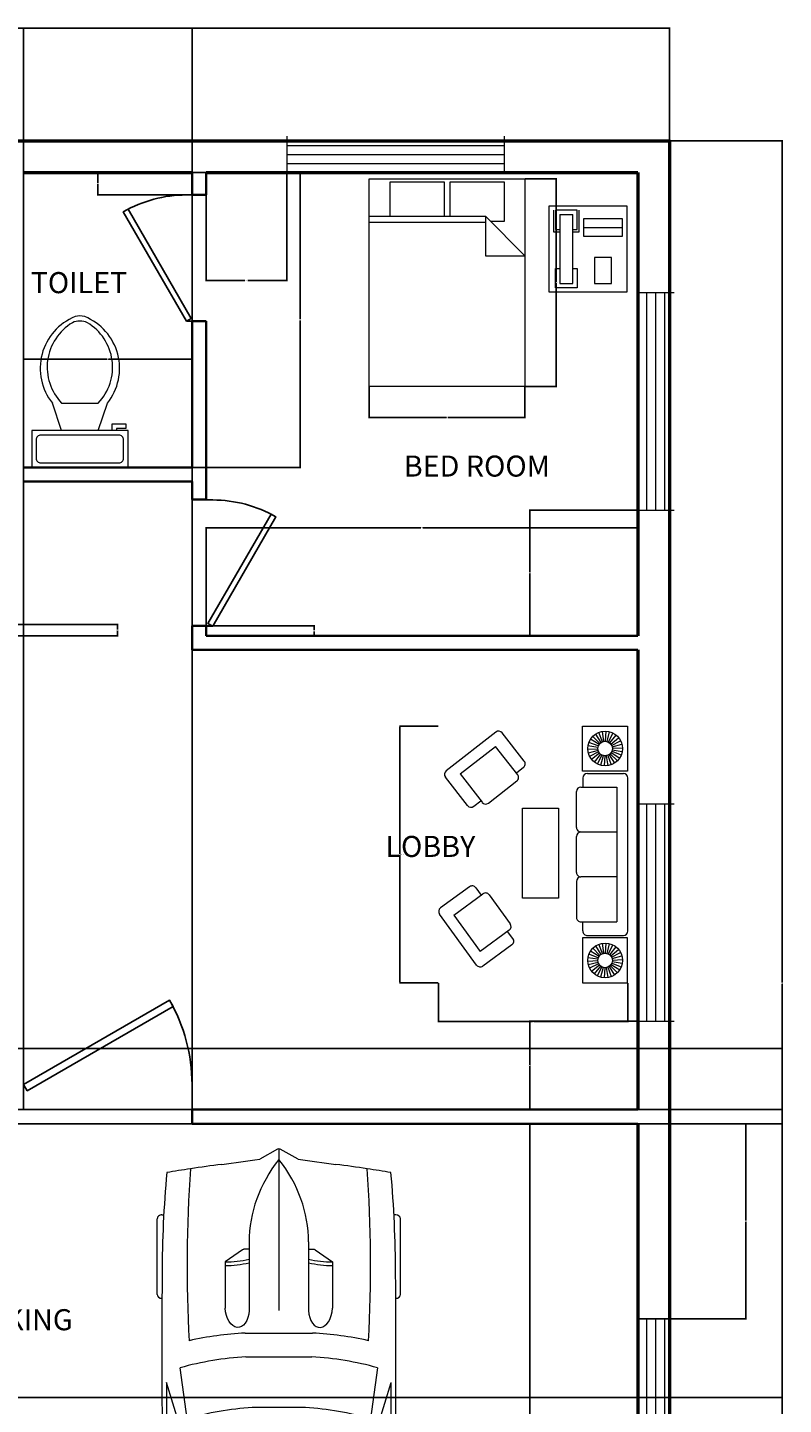
# Model space of a CAD drawing. Units: feet. Extents: x 3746 to 4170, y 1475 to 2148.
# Tile 5 of 5: x 3955 to 4170, y 1755 to 2148. Entities that reach past the tile are written whole.
import ezdxf

# ---------------------------------------------------------------- set-up
doc = ezdxf.new("R2010")
doc.units = ezdxf.units.FT
for name, color, linetype, lineweight in [('A-ANNO-DIMS', 2, 'Continuous', 18), ('A-AREA-IDEN', 7, 'Continuous', 25), ('A-EQPM', 8, 'Continuous', 13), ('A-FLOR-FIXT', 9, 'Continuous', 18), ('A-GLAZ', 91, 'Continuous', 18), ('CAR', 20, 'Continuous', 13), ('DOOR', 135, 'Continuous', 25), ('FURNITURE', 43, 'Continuous', 18), ('INWER WALL', 30, 'Continuous', 35), ('OUTER WALL', 31, 'Continuous', 50)]:
    doc.layers.add(name, color=color, linetype=linetype, lineweight=lineweight)
doc.styles.get("Standard").update_dxf_attribs({"font": 'arial.ttf'})
doc.dimstyles.get("Standard").update_dxf_attribs({"dimtxt": 0.18, "dimasz": 0.18, "dimexe": 0.18, "dimexo": 0.0625, "dimgap": 0.09, "dimtad": 0, "dimtih": 1, "dimtoh": 1, "dimdec": 4, "dimzin": 0, "dimdsep": 46, "dimtxsty": 'Standard', "dimcen": 0.09, "dimadec": 0, "dimazin": 0, "dimtfac": 1, "dimtdec": 4, "dimtofl": 0, "dimtmove": 0, "dimatfit": 3, "dimfxl": 1, "dimtolj": 1, "dimtzin": 0, "dimarcsym": 0})

# ---------------------------------------------------------------- blocks, each defined once
blk = doc.blocks.new('*U2')
for p, q in [((0, 0), (0, -6)), ((40, 0), (40, -6))]:
    blk.add_line(p, q)
blk.add_lwpolyline([(0, 0), (34.64, 20), (35.52, 18.48), (0.87, -1.52)], close=True)
blk.add_arc((0, 0), 40, 0, 30)
blk = doc.blocks.new('*U3')
for p, q in [((0, 0), (0, 6)), ((40, 0), (40, 6))]:
    blk.add_line(p, q)
blk.add_lwpolyline([(0, 0), (34.64, -20), (35.52, -18.48), (0.87, 1.52)], close=True)
blk.add_arc((0, 0), 40, 330, 0)
blk = doc.blocks.new('Bed - Queen')
for p, q in [((0, -80.00003), (0, 0)), ((0, 0), (59.99999, 0)), ((59.99999, 0), (59.99999, -80.00003)), ((7.99999, -1.2), (28.79998, -1.2)), ((7.99999, -14.4), (7.99999, -1.2)), ((28.79998, -1.2), (28.79998, -14.4)), ((31.19999, -1.2), (51.99999, -1.2)), ((31.19999, -14.4), (31.19999, -1.2)), ((51.99999, -1.2), (51.99999, -16.4)), ((0, -14.4), (44.8, -14.4)), ((59.99999, -29.6), (44.8, -14.4)), ((44.8, -14.4), (44.8, -29.6)), ((44.8, -16.8), (0, -16.8)), ((51.99999, -16.4), (46.79936, -16.4)), ((44.8, -29.6), (59.99999, -29.6)), ((59.99999, -80.00003), (0, -80.00003))]:
    blk.add_line(p, q)
blk = doc.blocks.new('Toilet - top')
for p, q in [((9.5, -6), (9.5, -2)), ((-10, -8.5), (-8, -8.5)), ((-10, -9.5), (-10, -8.5)), ((-8, -8.5), (-8, -8)), ((-7, -8), (-7, -9.5)), ((-4, -8), (-6, -14)), ((4, -8), (6, -14)), ((-7, -9.5), (-10, -9.5)), ((4, -14), (-4, -14))]:
    blk.add_line(p, q)
blk.add_lwpolyline([(10.5, -8), (10.5, 0), (-10.5, 0), (-10.5, -8)], close=True)
for points in [[(-9.5, -2), (-9.5, -6)], [(8.5, -1), (-8.5, -1)], [(-8.5, -7), (8.5, -7)]]:
    blk.add_lwpolyline(points)
for centre, radius, start, end in [((-8.62, -1.88), 0.884, 81.8699, 188.1301), ((8.62, -1.88), 0.884, 351.8699, 98.1301), ((-8.62, -6.12), 0.884, 171.8699, 278.1301), ((8.62, -6.12), 0.884, 261.8699, 8.1301), ((3.52, -21.58), 12.17, 141.4691, 247.9714), ((4.2, -21.82), 11.33, 136.3677, 238.9468), ((-3.52, -21.58), 12.17, 292.0284, 38.5307), ((-4.2, -21.82), 11.33, 301.053, 43.6321), ((0, -27.88), 4, 245.7318, 294.2682), ((0, -29), 4, 254.8605, 285.1395)]:
    blk.add_arc(centre, radius, start, end)
blk = doc.blocks.new('Phone - Desk')
for p, q in [((-4.5, -5), (-4.5, 5)), ((-4.5, 5), (4.5, 5)), ((4.5, 5), (4.5, -5)), ((-4, 4.5), (-4, 2)), ((-3.75, 4.5), (-3.75, 2.25)), ((-1.25, 4.5), (-3.75, 4.5)), ((-3.25, 4), (-3.25, -4)), ((-3.25, 4), (-1.75, 4)), ((-1.75, -4), (-1.75, 4)), ((-1.25, 2.25), (-1.25, 4.5)), ((-1, 2), (-1, 4.5)), ((4, 3.5), (-0.5, 3.5)), ((-0.5, 3.5), (-0.5, 1.5)), ((4, 1.5), (4, 3.5)), ((-4, 2), (-3.25, 2)), ((-3.75, 2.25), (-3.25, 2.25)), ((-1.75, 2.25), (-1.25, 2.25)), ((-1.75, 2), (-1, 2)), ((-0.5, 2.5), (4, 2.5)), ((-0.5, 1.5), (4, 1.5)), ((2.75, -1), (0.75, -1)), ((0.75, -1), (0.75, -4)), ((2.75, -4), (2.75, -1)), ((-3.75, -2.25), (-3.25, -2.25)), ((-3.75, -4.5), (-3.75, -2.25)), ((-1.75, -2.25), (-1.25, -2.25)), ((-1.25, -2.25), (-1.25, -4.5)), ((-1.25, -4.5), (-3.75, -4.5)), ((-3.25, -4), (-1.75, -4)), ((0.75, -4), (2.75, -4)), ((4.5, -5), (-4.5, -5))]:
    blk.add_line(p, q)
blk = doc.blocks.new('*U12')
for p, q in [((21.1, 37.41), (21.1, 36.83)), ((46.55, 38.89), (22.35, 38.89)), ((47.8, 37.39), (47.8, 37.41)), ((87.99, 31.87), (74.76, 35.92)), ((134.31, 35.6), (119.29, 31.78)), ((135.45, 37.07), (135.45, 37.41)), ((136.7, 38.89), (160.9, 38.89)), ((162.15, 37.41), (162.15, 36.77)), ((70.03, 31.54), (86.41, 29.35)), ((186.47, -33.5), (186.47, 33.5)), ((188.4, -32.76), (188.4, 32.76)), ((138.42, 29.35), (157.25, 29.35)), ((186.47, 29.35), (167.01, 29.35)), ((164.52, 26.39), (164.52, -26.39)), ((32.27, 11.63), (36.13, 17.17)), ((36.13, 17.17), (50.94, 17.17)), ((29.77, 9.51), (51.68, 9.51)), ((32.12, 9.51), (32.12, 11.15)), ((58.92, -10.77), (58.92, 10.77)), ((66.55, -10.53), (66.55, 10.53)), ((186.47, -10.53), (186.47, 10.53)), ((3.27, 6.13), (0.1, 0.41)), ((82.74, 8.5), (82.74, -8.5)), ((0, 0), (51.68, 0)), ((0.1, -0.41), (3.27, -6.13)), ((29.77, -9.51), (51.68, -9.51)), ((32.12, -9.51), (32.12, -11.15)), ((32.27, -11.63), (36.13, -17.17)), ((36.13, -17.17), (50.94, -17.17)), ((86.41, -29.35), (70.03, -31.54)), ((157.25, -29.35), (138.42, -29.35)), ((167.01, -29.35), (186.47, -29.35)), ((87.99, -31.87), (74.76, -35.92)), ((134.31, -35.6), (119.29, -31.78)), ((21.1, -37.41), (21.1, -36.83)), ((46.55, -38.89), (22.35, -38.89)), ((47.8, -37.39), (47.8, -37.41)), ((135.45, -37.07), (135.45, -37.41)), ((136.7, -38.89), (160.9, -38.89)), ((162.15, -37.41), (162.15, -36.77))]:
    blk.add_line(p, q)
for centre, major_axis, ratio, start_param, end_param in [((266.03, -27.52), (0, 313.31), 0.842304, 1.367076, 1.39176), ((41.19, -490.86), (0, 528.23), 0.842304, 0.00281, 0.075598), ((22.35, 37.41), (0, -1.48), 0.842304, 3.141593, 4.712389), ((64.48, -10555.62), (0, 10593.03), 0.842304, -0.013397, 0.002797), ((46.55, 37.41), (0, 1.48), 0.842304, -1.570796, 0), ((64.48, -10555.62), (0, -10591.55), 0.842304, 3.133765, 3.140441), ((136.7, 37.41), (0, -1.48), 0.842304, 3.141593, 4.712389), ((160.9, 37.41), (0, 1.48), 0.842304, -1.570796, 0), ((180.63, 35.84), (0, 2.22), 0.842304, -0.013017, 1.249894), ((64.48, -10556.36), (0, 10595.31), 0.842304, -0.013397, -0.013017), ((183.98, 33.5), (0, -2.96), 0.842304, 1.570796, 3.128196), ((183.98, 32.76), (0, -5.25), 0.842304, 1.570796, 3.128196), ((135.29, 5.39), (0, 81.77), 0.842304, 1.245306, 1.50788), ((95.79, -3666.35), (0, -3698.24), 0.842304, 3.134049, 3.144098), ((259.18, -27.52), (0, -305.3), 0.842304, 4.528606, 4.561838), ((37.47, -593.96), (0, -623.33), 0.842304, 3.096046, 3.200911), ((134.4, 5.39), (0, -89.78), 0.842304, 4.449482, 4.652344), ((149.6, 2.8), (0, -79.58), 0.842304, 4.372215, 4.640744), ((17.08, 0), (0, 147.02), 0.842304, 4.511394, 4.913384), ((35.91, 0), (0, 147.02), 0.842304, 4.511394, 4.913384), ((167.01, 26.39), (0, 2.96), 0.842304, 0, 1.570796), ((-204.49, 52.4), (0, -250.96), 0.842304, 1.385369, 1.434372), ((13.04, 17.01), (0, 27.42), 0.842304, 4.435146, 4.718221), ((14.2, 17.01), (0, 27.42), 0.842304, 4.435146, 4.718221), ((50.79, 13.34), (6.34, -0.36), 0.603834, -1.395552, 1.581315), ((29.77, -46.66), (0, 56.17), 0.842304, 0, 0.590319), ((32.75, 11.15), (0, 0.74), 0.842304, 0.879714, 1.570796), ((0.62, 0), (0, -0.74), 0.842304, 4.131459, 5.293319), ((29.77, 46.66), (0, 56.17), 0.842304, 2.551274, 3.141593), ((-204.49, -52.4), (0, 250.96), 0.842304, -1.434372, -1.385369), ((149.6, -2.8), (0, -79.58), 0.842304, -1.499151, -1.230623), ((32.75, -11.15), (0, -0.74), 0.842304, 4.712389, 5.403472), ((13.04, -17.01), (0, -27.42), 0.842304, 1.564964, 1.848039), ((14.2, -17.01), (0, -27.42), 0.842304, 1.564964, 1.848039), ((134.4, -5.39), (0, -89.78), 0.842304, -1.510751, -1.307889), ((135.29, -5.39), (0, -81.77), 0.842304, -1.50788, -1.245306), ((259.18, 27.52), (0, 305.3), 0.842304, 1.721348, 1.754579), ((167.01, -26.39), (0, -2.96), 0.842304, 4.712389, 6.283185), ((266.03, 27.52), (0, 313.31), 0.842304, 1.749832, 1.774517), ((37.47, 593.96), (0, -623.33), 0.842304, -0.059319, 0.045547), ((95.79, 3666.35), (0, -3698.24), 0.842304, -0.002505, 0.007544), ((183.98, -33.5), (0, 2.96), 0.842304, 3.15499, 4.712389), ((183.98, -32.76), (0, -5.25), 0.842304, 0.013397, 1.570796), ((41.19, 490.86), (0, -528.23), 0.842304, -0.075598, -0.00281), ((22.35, -37.41), (0, 1.48), 0.842304, 1.570796, 3.141593), ((64.48, 10555.62), (0, 10593.03), 0.842304, 3.138796, 3.15499), ((46.55, -37.41), (0, -1.48), 0.842304, 0, 1.570796), ((64.48, 10555.62), (0, -10591.55), 0.842304, 0.001152, 0.007828), ((136.7, -37.41), (0, -1.48), 0.842304, -1.570796, 0), ((160.9, -37.41), (0, 1.48), 0.842304, 3.141593, 4.712389), ((180.63, -35.84), (0, -2.22), 0.842304, -1.249894, 0.013017), ((64.48, 10556.36), (0, 10595.31), 0.842304, 3.15461, 3.15499)]:
    blk.add_ellipse(centre, major_axis=major_axis, ratio=ratio, start_param=start_param, end_param=end_param)
at = {"extrusion": (0, 0, -1)}
blk.add_ellipse((50.79, -13.34), major_axis=(6.34, 0.36), ratio=0.603834, start_param=-1.395552, end_param=1.581315, dxfattribs=at)
blk = doc.blocks.new('sofa arrangement 3')
for p, q in [((-912, 770), (-412, 770)), ((-912, 270), (-912, 770)), ((-412, 770), (-412, 270)), ((1365, 773), (-335, 773)), ((1443, 770), (1443, 270)), ((1943, 770), (1443, 770)), ((1943, 270), (1943, 770)), ((-725, 571), (-812, 641)), ((-713, 583), (-783, 670)), ((-698, 592), (-749, 692)), ((-682, 598), (-711, 706)), ((-665, 601), (-671, 712)), ((-648, 600), (-631, 710)), ((-633, 595), (-593, 700)), ((-618, 588), (-557, 682)), ((-604, 577), (-525, 656)), ((-594, 564), (-500, 625)), ((-385, 323), (-385, 723)), ((-235, 651), (1265, 651)), ((-235, 251), (-235, 651)), ((265, 251), (265, 651)), ((765, 651), (765, 251)), ((765, 651), (765, 251)), ((1265, 251), (1265, 651)), ((1415, 323), (1415, 723)), ((1630, 571), (1543, 641)), ((1642, 583), (1572, 670)), ((1656, 592), (1605, 692)), ((1672, 598), (1643, 706)), ((1689, 601), (1683, 712)), ((1706, 600), (1723, 710)), ((1722, 595), (1762, 700)), ((1737, 588), (1798, 682)), ((1750, 577), (1829, 656)), ((1761, 564), (1855, 625)), ((-743, 524), (-854, 530)), ((-742, 507), (-852, 490)), ((-740, 541), (-848, 570)), ((-737, 491), (-842, 451)), ((-734, 557), (-833, 607)), ((-730, 476), (-823, 415)), ((-719, 463), (-798, 383)), ((-599, 469), (-512, 398)), ((-589, 483), (-490, 432)), ((-586, 549), (-482, 589)), ((-583, 499), (-475, 470)), ((-582, 532), (-471, 550)), ((-581, 516), (-469, 510)), ((1612, 524), (1500, 530)), ((1613, 507), (1502, 490)), ((1615, 541), (1507, 570)), ((1617, 491), (1513, 451)), ((1621, 557), (1521, 607)), ((1625, 476), (1531, 415)), ((1636, 463), (1557, 383)), ((1756, 469), (1843, 398)), ((1765, 483), (1865, 432)), ((1769, 549), (1873, 589)), ((1771, 499), (1879, 470)), ((1773, 532), (1883, 550)), ((1774, 516), (1885, 510)), ((-706, 452), (-767, 358)), ((-691, 444), (-731, 340)), ((-674, 440), (-692, 329)), ((-657, 439), (-652, 327)), ((-641, 442), (-612, 333)), ((-625, 448), (-574, 348)), ((-611, 457), (-540, 370)), ((1649, 452), (1588, 358)), ((1664, 444), (1624, 340)), ((1680, 440), (1663, 329)), ((1697, 439), (1703, 327)), ((1714, 442), (1743, 333)), ((1730, 448), (1780, 348)), ((1744, 457), (1814, 370)), ((-412, 270), (-912, 270)), ((-335, 273), (-235, 273)), ((215, 201), (-185, 201)), ((715, 201), (315, 201)), ((815, 201), (1215, 201)), ((1365, 273), (1265, 273)), ((1443, 270), (1943, 270)), ((0, 0), (1000, 0)), ((0, -400), (0, 0)), ((1000, 0), (1000, -400)), ((-521, -378), (-836, -624)), ((-372, -452), (-687, -698)), ((-451, -387), (-390, -466)), ((1000, -400), (0, -400)), ((-56, -776), (-302, -461)), ((963, -770), (1286, -534)), ((1356, -545), (1592, -869)), ((1450, -505), (1370, -564)), ((1520, -516), (1756, -838)), ((-845, -694), (-415, -1246)), ((-380, -1092), (-687, -698)), ((-380, -1092), (-65, -847)), ((-380, -1092), (-65, -847)), ((-21, -939), (-82, -861)), ((885, -917), (966, -858)), ((1188, -1163), (952, -840)), ((1188, -1163), (952, -840)), ((1745, -908), (1179, -1321)), ((1188, -1163), (1592, -869)), ((-30, -1010), (-345, -1255)), ((874, -987), (1109, -1310))]:
    blk.add_line(p, q)
for centre, radius in [((-662, 520), 193), ((1692, 520), 193), ((-662, 520), 81), ((1693, 520), 81)]:
    blk.add_circle(centre, radius)
for centre, start, end in [((-335, 723), 90, 180), ((1365, 723), 0, 90), ((-335, 323), 180, 270), ((1365, 323), 270, 0), ((-185, 251), 180, 270), ((215, 251), 270, 0), ((315, 251), 180, 270), ((715, 251), 270, 0), ((815, 251), 180, 270), ((1215, 251), 270, 0), ((-491, -418), 37.9081, 127.9081), ((-341, -492), 37.9081, 127.9081), ((1316, -575), 36.0842, 126.0842), ((1480, -545), 36.0842, 126.0842), ((-806, -663), 127.9081, 217.9081), ((-95, -807), 307.9081, 37.9081), ((914, -958), 126.0842, 216.0842), ((993, -810), 126.0842, 216.0842), ((1715, -868), 306.0842, 36.0842), ((-60, -970), 307.9081, 37.9081), ((-375, -1216), 217.9081, 307.9081), ((1149, -1280), 216.0842, 306.0842)]:
    blk.add_arc(centre, 50, start, end)
blk = doc.blocks.new('Window - Wood Frame 36 in. Wide plan')
for p, q in [((0, 6), (0, 0)), ((36, 6), (36, 0)), ((0, 4.5), (36, 4.5)), ((0, 3), (36, 3)), ((0, 1.5), (36, 1.5))]:
    blk.add_line(p, q)
blk = doc.blocks.new('*D39')
at = {"layer": 'A-ANNO-DIMS', "color": 0, "lineweight": -2, "transparency": 16777216}
for p, q in [((4096.36, 2104.57), (4105.34, 2104.57)), ((4105.16, 2104.39), (4105.16, 2075.18)), ((4105.16, 2045.61), (4105.16, 2074.82)), ((4096.36, 2045.43), (4105.34, 2045.43))]:
    blk.add_line(p, q, dxfattribs=at)
at = {"layer": 'A-ANNO-DIMS', "color": 0, "transparency": 16777216}
for points in [[(4105.13, 2104.39), (4105.19, 2104.39), (4105.16, 2104.57)], [(4105.13, 2045.61), (4105.19, 2045.61), (4105.16, 2045.43)]]:
    blk.add_solid(points, dxfattribs=at)
at = {"layer": 'Defpoints', "color": 0, "transparency": 16777216}
for p in [(4096.29, 2104.57), (4105.16, 2104.57), (4096.29, 2045.43)]:
    blk.add_point(p, dxfattribs=at)
at = {"layer": 'A-ANNO-DIMS', "color": 0, "transparency": 16777216, "insert": (4105.16, 2075), "char_height": 0.18, "attachment_point": 5}
blk.add_mtext('\\A1;BED 59', dxfattribs=at)
blk = doc.blocks.new('*D40')
at = {"layer": 'A-ANNO-DIMS', "color": 0, "lineweight": -2, "transparency": 16777216}
for p, q in [((4051.94, 2045.37), (4051.94, 2036.38)), ((4096.29, 2045.37), (4096.29, 2036.38)), ((4052.12, 2036.56), (4073.89, 2036.56)), ((4096.11, 2036.56), (4074.34, 2036.56))]:
    blk.add_line(p, q, dxfattribs=at)
at = {"layer": 'A-ANNO-DIMS', "color": 0, "transparency": 16777216}
for points in [[(4052.12, 2036.59), (4052.12, 2036.53), (4051.94, 2036.56)], [(4096.11, 2036.59), (4096.11, 2036.53), (4096.29, 2036.56)]]:
    blk.add_solid(points, dxfattribs=at)
at = {"layer": 'Defpoints', "color": 0, "transparency": 16777216}
for p in [(4051.94, 2045.43), (4096.29, 2045.43), (4096.29, 2036.56)]:
    blk.add_point(p, dxfattribs=at)
at = {"layer": 'A-ANNO-DIMS', "color": 0, "transparency": 16777216, "insert": (4074.11, 2036.56), "char_height": 0.18, "attachment_point": 5}
blk.add_mtext('\\A1;44', dxfattribs=at)
blk = doc.blocks.new('*D53')
at = {"layer": 'A-ANNO-DIMS', "color": 0, "lineweight": -2, "transparency": 16777216}
for p, q in [((4071.59, 1948.65), (4060.5, 1948.65)), ((4060.68, 1948.47), (4060.68, 1912.25)), ((4060.68, 1875.66), (4060.68, 1911.88)), ((4071.59, 1875.48), (4060.5, 1875.48))]:
    blk.add_line(p, q, dxfattribs=at)
at = {"layer": 'A-ANNO-DIMS', "color": 0, "transparency": 16777216}
for points in [[(4060.65, 1948.47), (4060.71, 1948.47), (4060.68, 1948.65)], [(4060.65, 1875.66), (4060.71, 1875.66), (4060.68, 1875.48)]]:
    blk.add_solid(points, dxfattribs=at)
at = {"layer": 'Defpoints', "color": 0, "transparency": 16777216}
for p in [(4071.66, 1948.65), (4060.68, 1875.48), (4071.66, 1875.48)]:
    blk.add_point(p, dxfattribs=at)
at = {"layer": 'A-ANNO-DIMS', "color": 0, "transparency": 16777216, "insert": (4060.68, 1912.06), "char_height": 0.18, "attachment_point": 5}
blk.add_mtext('\\A1;SEATING GROUP 73', dxfattribs=at)
blk = doc.blocks.new('*D54')
at = {"layer": 'A-ANNO-DIMS', "color": 0, "lineweight": -2, "transparency": 16777216}
for p, q in [((4071.66, 1875.42), (4071.66, 1864.32)), ((4125.6, 1875.42), (4125.6, 1864.32)), ((4071.84, 1864.5), (4098.41, 1864.5)), ((4125.42, 1864.5), (4098.85, 1864.5))]:
    blk.add_line(p, q, dxfattribs=at)
at = {"layer": 'A-ANNO-DIMS', "color": 0, "transparency": 16777216}
for points in [[(4071.84, 1864.53), (4071.84, 1864.47), (4071.66, 1864.5)], [(4125.42, 1864.53), (4125.42, 1864.47), (4125.6, 1864.5)]]:
    blk.add_solid(points, dxfattribs=at)
at = {"layer": 'Defpoints', "color": 0, "transparency": 16777216}
for p in [(4071.66, 1875.48), (4125.6, 1875.48), (4125.6, 1864.5)]:
    blk.add_point(p, dxfattribs=at)
at = {"layer": 'A-ANNO-DIMS', "color": 0, "transparency": 16777216, "insert": (4098.63, 1864.5), "char_height": 0.18, "attachment_point": 5}
blk.add_mtext('\\A1;54', dxfattribs=at)
blk = doc.blocks.new('*D55')
at = {"layer": 'A-ANNO-DIMS', "color": 0, "lineweight": -2, "transparency": 16777216}
for p, q in [((3777.43, 2115.45), (3777.43, 2147.69)), ((3777.61, 2147.51), (3957.14, 2147.51)), ((4137.25, 2147.51), (3957.72, 2147.51)), ((4137.43, 2115.45), (4137.43, 2147.69))]:
    blk.add_line(p, q, dxfattribs=at)
at = {"layer": 'A-ANNO-DIMS', "color": 0, "transparency": 16777216}
for points in [[(3777.61, 2147.54), (3777.61, 2147.48), (3777.43, 2147.51)], [(4137.25, 2147.54), (4137.25, 2147.48), (4137.43, 2147.51)]]:
    blk.add_solid(points, dxfattribs=at)
at = {"layer": 'Defpoints', "color": 0, "transparency": 16777216}
for p in [(4137.43, 2147.51), (3777.43, 2115.38), (4137.43, 2115.38)]:
    blk.add_point(p, dxfattribs=at)
at = {"layer": 'A-ANNO-DIMS', "color": 0, "transparency": 16777216, "insert": (3957.43, 2147.51), "char_height": 0.18, "attachment_point": 5}
blk.add_mtext('\\A1;360', dxfattribs=at)
blk = doc.blocks.new('*D56')
at = {"layer": 'A-ANNO-DIMS', "color": 0, "lineweight": -2, "transparency": 16777216}
for p, q in [((4137.49, 2115.38), (4169.74, 2115.38)), ((4169.56, 2115.2), (4169.56, 1875.56)), ((4169.56, 1635.56), (4169.56, 1875.2)), ((4137.49, 1635.38), (4169.74, 1635.38))]:
    blk.add_line(p, q, dxfattribs=at)
at = {"layer": 'A-ANNO-DIMS', "color": 0, "transparency": 16777216}
for points in [[(4169.53, 2115.2), (4169.59, 2115.2), (4169.56, 2115.38)], [(4169.53, 1635.56), (4169.59, 1635.56), (4169.56, 1635.38)]]:
    blk.add_solid(points, dxfattribs=at)
at = {"layer": 'Defpoints', "color": 0, "transparency": 16777216}
for p in [(4137.43, 2115.38), (4137.43, 1635.38), (4169.56, 1635.38)]:
    blk.add_point(p, dxfattribs=at)
at = {"layer": 'A-ANNO-DIMS', "color": 0, "transparency": 16777216, "insert": (4169.56, 1875.38), "char_height": 0.18, "attachment_point": 5}
blk.add_mtext('\\A1;480', dxfattribs=at)
blk = doc.blocks.new('*D58')
at = {"layer": 'A-ANNO-DIMS', "color": 0, "lineweight": -2, "transparency": 16777216}
for p, q in [((3953.43, 2022.45), (3953.43, 2053.36)), ((3953.61, 2053.18), (3977.21, 2053.18)), ((4001.25, 2053.18), (3977.65, 2053.18)), ((4001.43, 2022.45), (4001.43, 2053.36))]:
    blk.add_line(p, q, dxfattribs=at)
at = {"layer": 'A-ANNO-DIMS', "color": 0, "transparency": 16777216}
for points in [[(3953.61, 2053.21), (3953.61, 2053.15), (3953.43, 2053.18)], [(4001.25, 2053.21), (4001.25, 2053.15), (4001.43, 2053.18)]]:
    blk.add_solid(points, dxfattribs=at)
at = {"layer": 'Defpoints', "color": 0, "transparency": 16777216}
for p in [(4001.43, 2053.18), (3953.43, 2022.38), (4001.43, 2022.38)]:
    blk.add_point(p, dxfattribs=at)
at = {"layer": 'A-ANNO-DIMS', "color": 0, "transparency": 16777216, "insert": (3977.43, 2053.18), "char_height": 0.18, "attachment_point": 5}
blk.add_mtext('\\A1;48', dxfattribs=at)
blk = doc.blocks.new('*D59')
at = {"layer": 'A-ANNO-DIMS', "color": 0, "lineweight": -2, "transparency": 16777216}
for p, q in [((4005.43, 1974.45), (4005.43, 2005.36)), ((4005.61, 2005.18), (4066.65, 2005.18)), ((4128.25, 2005.18), (4067.21, 2005.18)), ((4128.43, 1974.45), (4128.43, 2005.36))]:
    blk.add_line(p, q, dxfattribs=at)
at = {"layer": 'A-ANNO-DIMS', "color": 0, "transparency": 16777216}
for points in [[(4005.61, 2005.21), (4005.61, 2005.15), (4005.43, 2005.18)], [(4128.25, 2005.21), (4128.25, 2005.15), (4128.43, 2005.18)]]:
    blk.add_solid(points, dxfattribs=at)
at = {"layer": 'Defpoints', "color": 0, "transparency": 16777216}
for p in [(4128.43, 2005.18), (4005.43, 1974.38), (4128.43, 1974.38)]:
    blk.add_point(p, dxfattribs=at)
at = {"layer": 'A-ANNO-DIMS', "color": 0, "transparency": 16777216, "insert": (4066.93, 2005.18), "char_height": 0.18, "attachment_point": 5}
blk.add_mtext('\\A1;123', dxfattribs=at)
blk = doc.blocks.new('*D61')
at = {"layer": 'A-ANNO-DIMS', "color": 0, "lineweight": -2, "transparency": 16777216}
for p, q in [((4001.49, 2106.38), (4032.41, 2106.38)), ((4032.23, 2106.2), (4032.23, 2064.56)), ((4032.23, 2022.56), (4032.23, 2064.2)), ((4001.49, 2022.38), (4032.41, 2022.38))]:
    blk.add_line(p, q, dxfattribs=at)
at = {"layer": 'A-ANNO-DIMS', "color": 0, "transparency": 16777216}
for points in [[(4032.2, 2106.2), (4032.26, 2106.2), (4032.23, 2106.38)], [(4032.2, 2022.56), (4032.26, 2022.56), (4032.23, 2022.38)]]:
    blk.add_solid(points, dxfattribs=at)
at = {"layer": 'Defpoints', "color": 0, "transparency": 16777216}
for p in [(4001.43, 2106.38), (4001.43, 2022.38), (4032.23, 2022.38)]:
    blk.add_point(p, dxfattribs=at)
at = {"layer": 'A-ANNO-DIMS', "color": 0, "transparency": 16777216, "insert": (4032.23, 2064.38), "char_height": 0.18, "attachment_point": 5}
blk.add_mtext('\\A1;84', dxfattribs=at)
blk = doc.blocks.new('*D67')
at = {"layer": 'A-ANNO-DIMS', "color": 0, "lineweight": -2, "transparency": 16777216}
for p, q in [((3902.49, 1835.38), (4169.74, 1835.38)), ((4169.56, 1835.2), (4169.56, 1796.56)), ((4169.56, 1757.56), (4169.56, 1796.2)), ((3902.49, 1757.38), (4169.74, 1757.38))]:
    blk.add_line(p, q, dxfattribs=at)
at = {"layer": 'A-ANNO-DIMS', "color": 0, "transparency": 16777216}
for points in [[(4169.53, 1835.2), (4169.59, 1835.2), (4169.56, 1835.38)], [(4169.53, 1757.56), (4169.59, 1757.56), (4169.56, 1757.38)]]:
    blk.add_solid(points, dxfattribs=at)
at = {"layer": 'Defpoints', "color": 0, "transparency": 16777216}
for p in [(3902.43, 1835.38), (3902.43, 1757.38), (4169.56, 1757.38)]:
    blk.add_point(p, dxfattribs=at)
at = {"layer": 'A-ANNO-DIMS', "color": 0, "transparency": 16777216, "insert": (4169.56, 1796.38), "char_height": 0.18, "attachment_point": 5}
blk.add_mtext('\\A1;78', dxfattribs=at)
blk = doc.blocks.new('*D72')
at = {"layer": 'A-ANNO-DIMS', "color": 0, "lineweight": -2, "transparency": 16777216}
for p, q in [((4128.37, 1835.38), (4097.45, 1835.38)), ((4097.63, 1835.2), (4097.63, 1740.06)), ((4097.63, 1644.56), (4097.63, 1739.7)), ((4128.37, 1644.38), (4097.45, 1644.38))]:
    blk.add_line(p, q, dxfattribs=at)
at = {"layer": 'A-ANNO-DIMS', "color": 0, "transparency": 16777216}
for points in [[(4097.6, 1835.2), (4097.66, 1835.2), (4097.63, 1835.38)], [(4097.6, 1644.56), (4097.66, 1644.56), (4097.63, 1644.38)]]:
    blk.add_solid(points, dxfattribs=at)
at = {"layer": 'Defpoints', "color": 0, "transparency": 16777216}
for p in [(4097.63, 1835.38), (4128.43, 1835.38), (4128.43, 1644.38)]:
    blk.add_point(p, dxfattribs=at)
at = {"layer": 'A-ANNO-DIMS', "color": 0, "transparency": 16777216, "insert": (4097.63, 1739.88), "char_height": 0.18, "attachment_point": 5}
blk.add_mtext('\\A1;191', dxfattribs=at)
blk = doc.blocks.new('*D77')
at = {"layer": 'A-ANNO-DIMS', "color": 0, "lineweight": -2, "transparency": 16777216}
for p, q in [((3953.43, 1839.45), (3953.43, 2147.69)), ((3953.61, 2147.51), (3977.21, 2147.51)), ((4001.25, 2147.51), (3977.65, 2147.51)), ((4001.43, 1839.45), (4001.43, 2147.69))]:
    blk.add_line(p, q, dxfattribs=at)
at = {"layer": 'A-ANNO-DIMS', "color": 0, "transparency": 16777216}
for points in [[(3953.61, 2147.54), (3953.61, 2147.48), (3953.43, 2147.51)], [(4001.25, 2147.54), (4001.25, 2147.48), (4001.43, 2147.51)]]:
    blk.add_solid(points, dxfattribs=at)
at = {"layer": 'Defpoints', "color": 0, "transparency": 16777216}
for p in [(4001.43, 2147.51), (3953.43, 1839.38), (4001.43, 1839.38)]:
    blk.add_point(p, dxfattribs=at)
at = {"layer": 'A-ANNO-DIMS', "color": 0, "transparency": 16777216, "insert": (3977.43, 2147.51), "char_height": 0.18, "attachment_point": 5}
blk.add_mtext('\\A1;48', dxfattribs=at)
blk = doc.blocks.new('*D81')
at = {"layer": 'A-ANNO-DIMS', "color": 0, "lineweight": -2, "transparency": 16777216}
for p, q in [((4005.43, 2106.32), (4005.43, 2075.4)), ((4028.41, 2106.32), (4028.41, 2075.4)), ((4005.61, 2075.58), (4016.52, 2075.58)), ((4028.23, 2075.58), (4017.32, 2075.58))]:
    blk.add_line(p, q, dxfattribs=at)
at = {"layer": 'A-ANNO-DIMS', "color": 0, "transparency": 16777216}
for points in [[(4005.61, 2075.61), (4005.61, 2075.55), (4005.43, 2075.58)], [(4028.23, 2075.61), (4028.23, 2075.55), (4028.41, 2075.58)]]:
    blk.add_solid(points, dxfattribs=at)
at = {"layer": 'Defpoints', "color": 0, "transparency": 16777216}
for p in [(4005.43, 2106.38), (4028.41, 2106.38), (4005.43, 2075.58)]:
    blk.add_point(p, dxfattribs=at)
at = {"layer": 'A-ANNO-DIMS', "color": 0, "transparency": 16777216, "insert": (4016.92, 2075.58), "char_height": 0.18, "attachment_point": 5}
blk.add_mtext('\\A1;22.98', dxfattribs=at)
blk = doc.blocks.new('*D83')
at = {"layer": 'A-ANNO-DIMS', "color": 0, "lineweight": -2, "transparency": 16777216}
for p, q in [((4128.37, 2010.22), (4097.45, 2010.22)), ((4097.63, 2010.04), (4097.63, 1992.48)), ((4097.63, 1974.56), (4097.63, 1992.12)), ((4128.37, 1974.38), (4097.45, 1974.38))]:
    blk.add_line(p, q, dxfattribs=at)
at = {"layer": 'A-ANNO-DIMS', "color": 0, "transparency": 16777216}
for points in [[(4097.6, 2010.04), (4097.66, 2010.04), (4097.63, 2010.22)], [(4097.6, 1974.56), (4097.66, 1974.56), (4097.63, 1974.38)]]:
    blk.add_solid(points, dxfattribs=at)
at = {"layer": 'Defpoints', "color": 0, "transparency": 16777216}
for p in [(4097.63, 2010.22), (4128.43, 2010.22), (4128.43, 1974.38)]:
    blk.add_point(p, dxfattribs=at)
at = {"layer": 'A-ANNO-DIMS', "color": 0, "transparency": 16777216, "insert": (4097.63, 1992.3), "char_height": 0.18, "attachment_point": 5}
blk.add_mtext('\\A1;35.84', dxfattribs=at)
blk = doc.blocks.new('*D84')
at = {"layer": 'A-ANNO-DIMS', "color": 0, "lineweight": -2, "transparency": 16777216}
for p, q in [((4128.37, 1864.59), (4097.45, 1864.59)), ((4097.63, 1864.41), (4097.63, 1852.17)), ((4097.63, 1839.56), (4097.63, 1851.8)), ((4128.37, 1839.38), (4097.45, 1839.38))]:
    blk.add_line(p, q, dxfattribs=at)
at = {"layer": 'A-ANNO-DIMS', "color": 0, "transparency": 16777216}
for points in [[(4097.6, 1864.41), (4097.66, 1864.41), (4097.63, 1864.59)], [(4097.6, 1839.56), (4097.66, 1839.56), (4097.63, 1839.38)]]:
    blk.add_solid(points, dxfattribs=at)
at = {"layer": 'Defpoints', "color": 0, "transparency": 16777216}
for p in [(4097.63, 1864.59), (4128.43, 1864.59), (4128.43, 1839.38)]:
    blk.add_point(p, dxfattribs=at)
at = {"layer": 'A-ANNO-DIMS', "color": 0, "transparency": 16777216, "insert": (4097.63, 1851.98), "char_height": 0.18, "attachment_point": 5}
blk.add_mtext('\\A1;25.204', dxfattribs=at)
blk = doc.blocks.new('*D85')
at = {"layer": 'A-ANNO-DIMS', "color": 0, "lineweight": -2, "transparency": 16777216}
for p, q in [((4128.49, 1835.38), (4159.41, 1835.38)), ((4159.23, 1835.2), (4159.23, 1807.76)), ((4159.23, 1779.95), (4159.23, 1807.4)), ((4128.49, 1779.77), (4159.41, 1779.77))]:
    blk.add_line(p, q, dxfattribs=at)
at = {"layer": 'A-ANNO-DIMS', "color": 0, "transparency": 16777216}
for points in [[(4159.2, 1835.2), (4159.26, 1835.2), (4159.23, 1835.38)], [(4159.2, 1779.95), (4159.26, 1779.95), (4159.23, 1779.77)]]:
    blk.add_solid(points, dxfattribs=at)
at = {"layer": 'Defpoints', "color": 0, "transparency": 16777216}
for p in [(4128.43, 1835.38), (4128.43, 1779.77), (4159.23, 1779.77)]:
    blk.add_point(p, dxfattribs=at)
at = {"layer": 'A-ANNO-DIMS', "color": 0, "transparency": 16777216, "insert": (4159.23, 1807.58), "char_height": 0.18, "attachment_point": 5}
blk.add_mtext('\\A1;55.61', dxfattribs=at)
blk = doc.blocks.new('*D89')
at = {"layer": 'A-ANNO-DIMS', "color": 0, "lineweight": -2, "transparency": 16777216}
for p, q in [((3906.49, 1856.82), (4169.74, 1856.82)), ((4169.56, 1856.64), (4169.56, 1848.28)), ((4169.56, 1839.56), (4169.56, 1847.92)), ((3906.49, 1839.38), (4169.74, 1839.38))]:
    blk.add_line(p, q, dxfattribs=at)
at = {"layer": 'A-ANNO-DIMS', "color": 0, "transparency": 16777216}
for points in [[(4169.53, 1856.64), (4169.59, 1856.64), (4169.56, 1856.82)], [(4169.53, 1839.56), (4169.59, 1839.56), (4169.56, 1839.38)]]:
    blk.add_solid(points, dxfattribs=at)
at = {"layer": 'Defpoints', "color": 0, "transparency": 16777216}
for p in [(3906.43, 1856.82), (4169.56, 1856.82), (3906.43, 1839.38)]:
    blk.add_point(p, dxfattribs=at)
at = {"layer": 'A-ANNO-DIMS', "color": 0, "transparency": 16777216, "insert": (4169.56, 1848.1), "char_height": 0.18, "attachment_point": 5}
blk.add_mtext('\\A1;17.442', dxfattribs=at)
blk = doc.blocks.new('*D90')
at = {"layer": 'A-ANNO-DIMS', "color": 0, "lineweight": -2, "transparency": 16777216}
for p, q in [((3949.49, 1977.56), (3980.41, 1977.56)), ((3980.23, 1977.38), (3980.23, 1976.15)), ((3949.49, 1974.38), (3980.41, 1974.38)), ((3980.23, 1974.56), (3980.23, 1975.79))]:
    blk.add_line(p, q, dxfattribs=at)
at = {"layer": 'A-ANNO-DIMS', "color": 0, "transparency": 16777216}
for points in [[(3980.2, 1977.38), (3980.26, 1977.38), (3980.23, 1977.56)], [(3980.2, 1974.56), (3980.26, 1974.56), (3980.23, 1974.38)]]:
    blk.add_solid(points, dxfattribs=at)
at = {"layer": 'Defpoints', "color": 0, "transparency": 16777216}
for p in [(3949.43, 1977.56), (3949.43, 1974.38), (3980.23, 1974.38)]:
    blk.add_point(p, dxfattribs=at)
at = {"layer": 'A-ANNO-DIMS', "color": 0, "transparency": 16777216, "insert": (3980.23, 1975.97), "char_height": 0.18, "attachment_point": 5}
blk.add_mtext('\\A1;3.18', dxfattribs=at)
blk = doc.blocks.new('*D91')
at = {"layer": 'A-ANNO-DIMS', "color": 0, "lineweight": -2, "transparency": 16777216}
for p, q in [((4005.49, 1977.21), (4036.41, 1977.21)), ((4005.49, 1974.38), (4036.41, 1974.38)), ((4036.23, 1977.03), (4036.23, 1975.98)), ((4036.23, 1974.56), (4036.23, 1975.61))]:
    blk.add_line(p, q, dxfattribs=at)
at = {"layer": 'A-ANNO-DIMS', "color": 0, "transparency": 16777216}
for points in [[(4036.2, 1977.03), (4036.26, 1977.03), (4036.23, 1977.21)], [(4036.2, 1974.56), (4036.26, 1974.56), (4036.23, 1974.38)]]:
    blk.add_solid(points, dxfattribs=at)
at = {"layer": 'Defpoints', "color": 0, "transparency": 16777216}
for p in [(4005.43, 1977.21), (4005.43, 1974.38), (4036.23, 1974.38)]:
    blk.add_point(p, dxfattribs=at)
at = {"layer": 'A-ANNO-DIMS', "color": 0, "transparency": 16777216, "insert": (4036.23, 1975.8), "char_height": 0.18, "attachment_point": 5}
blk.add_mtext('\\A1;2.828', dxfattribs=at)
blk = doc.blocks.new('*D92')
at = {"layer": 'A-ANNO-DIMS', "color": 0, "lineweight": -2, "transparency": 16777216}
for p, q in [((4005.37, 2106.38), (3974.45, 2106.38)), ((3974.63, 2106.2), (3974.63, 2103.39)), ((3974.63, 2100.22), (3974.63, 2103.03)), ((4005.37, 2100.04), (3974.45, 2100.04))]:
    blk.add_line(p, q, dxfattribs=at)
at = {"layer": 'A-ANNO-DIMS', "color": 0, "transparency": 16777216}
for points in [[(3974.6, 2106.2), (3974.66, 2106.2), (3974.63, 2106.38)], [(3974.6, 2100.22), (3974.66, 2100.22), (3974.63, 2100.04)]]:
    blk.add_solid(points, dxfattribs=at)
at = {"layer": 'Defpoints', "color": 0, "transparency": 16777216}
for p in [(3974.63, 2106.38), (4005.43, 2106.38), (4005.43, 2100.04)]:
    blk.add_point(p, dxfattribs=at)
at = {"layer": 'A-ANNO-DIMS', "color": 0, "transparency": 16777216, "insert": (3974.63, 2103.21), "char_height": 0.18, "attachment_point": 5}
blk.add_mtext('\\A1;6.344', dxfattribs=at)

msp = doc.modelspace()

# ---------------------------------------------------------------- linework, layer by layer
at = {"layer": 'INWER WALL'}
for p, q in [((4001.4289, 2106.3828), (4001.4289, 2100.039)), ((4005.4289, 2106.3828), (4005.4289, 2100.039)), ((4001.4289, 2100.039), (4005.4289, 2100.039)), ((4001.4289, 2064.039), (4005.4289, 2064.039)), ((4001.4289, 2064.039), (4001.4289, 2022.3828)), ((4005.4289, 2064.039), (4005.4289, 2013.2106)), ((3953.4289, 2022.3828), (4001.4289, 2022.3828)), ((3953.4289, 2018.3828), (4001.4289, 2018.3828)), ((4001.4289, 2018.3828), (4001.4289, 2013.2106)), ((4001.4289, 2013.2106), (4005.4289, 2013.2106)), ((4001.4289, 1977.2106), (4005.4289, 1977.2106)), ((4001.4289, 1977.2106), (4001.4289, 1970.3828)), ((4005.4289, 1977.2106), (4005.4289, 1974.3828)), ((4005.4289, 1974.3828), (4128.4289, 1974.3828)), ((4001.4289, 1970.3828), (4128.4289, 1970.3828)), ((4001.4289, 1839.3828), (4001.4289, 1835.3828)), ((4001.4289, 1839.3828), (4128.4289, 1839.3828)), ((4001.4289, 1835.3828), (4128.4289, 1835.3828))]:
    msp.add_line(p, q, dxfattribs=at)
at = {"layer": 'OUTER WALL'}
for p, q in [((3953.4289, 2106.3828), (4001.4289, 2106.3828)), ((4005.4289, 2106.3828), (4128.4289, 2106.3828)), ((4128.4289, 2106.3828), (4128.4289, 1974.3828)), ((4128.4289, 1970.3828), (4128.4289, 1839.3828)), ((4128.4289, 1835.3828), (4128.4289, 1644.3828))]:
    msp.add_line(p, q, dxfattribs=at)
msp.add_lwpolyline([(3948.7526, 1635.3828), (3777.4289, 1635.3828), (3777.4289, 2115.3828), (4137.4289, 2115.3828), (4137.4289, 1635.3828), (4068.7526, 1635.3828)], dxfattribs=at)

# ---------------------------------------------------------------- block references
at = {"layer": 'A-EQPM', "xscale": 2.45986272692771, "yscale": 2.45986272692771, "zscale": 2.45986272692771}
msp.add_blockref('Phone - Desk', (4114.215, 2084.598), dxfattribs=at)
at = {"layer": 'A-FLOR-FIXT', "xscale": 1.307475105199699, "yscale": 1.307475105199699, "zscale": 1.307475105199699, "rotation": 180}
msp.add_blockref('Toilet - top', (3969.4812, 2022.3747), dxfattribs=at)
at = {"layer": 'A-GLAZ', "xscale": 1.721338572628536, "yscale": 1.721338572628536, "zscale": 1.721338572628536}
msp.add_blockref('Window - Wood Frame 36 in. Wide plan', (4028.4106, 2106.3828), dxfattribs=at)
at = {"layer": 'A-GLAZ', "xscale": 1.721338572628536, "yscale": 1.721338572628536, "zscale": 1.721338572628536, "rotation": 90}
for p in [(4138.7569, 2010.2222), (4138.7569, 1864.5866), (4138.7569, 1717.8058)]:
    msp.add_blockref('Window - Wood Frame 36 in. Wide plan', p, dxfattribs=at)
at = {"layer": 'CAR', "xscale": 0.890498965628364, "yscale": 0.890498965628364, "zscale": 0.890498965628364, "rotation": 270}
msp.add_blockref('*U12', (4026.167, 1828.1892), dxfattribs=at)
at = {"layer": 'DOOR', "xscale": 0.9000000000000054, "yscale": 0.9000000000000054, "zscale": 0.9000000000000054, "rotation": 90}
for name, p in [('*U2', (3999.8507, 2063.986)), ('*U3', (4007.3326, 1977.0848))]:
    msp.add_blockref(name, p, dxfattribs=at)
at = {"layer": 'DOOR', "xscale": 1.200000000000002, "yscale": 1.200000000000002, "zscale": 1.200000000000002}
msp.add_blockref('*U2', (3953.4289, 1846.5828), dxfattribs=at)
at = {"layer": 'FURNITURE', "xscale": 0.7392717418392168, "yscale": 0.7392717418392168, "zscale": 0.7392717418392168}
msp.add_blockref('Bed - Queen', (4051.9367, 2104.5712), dxfattribs=at)
at = {"layer": 'FURNITURE', "xscale": 0.0256327584730773, "yscale": 0.0256327584730773, "zscale": 0.0256327584730773, "rotation": 270}
msp.add_blockref('sofa arrangement 3', (4105.793, 1925.2814), dxfattribs=at)

# ---------------------------------------------------------------- texts
at = {"layer": 'A-AREA-IDEN', "char_height": 6, "attachment_point": 1}
for s, heights, insert in [('TOILET', [0], (3955.4542, 2078.0101)), ('\\pxt8;BED ROOM', [0], (4061.7667, 2025.7455)), ('LOBBY', [6.2087], (4056.5319, 1917.374)), ('PARKING', [0], (3932.8141, 1782.5296))]:
    msp.add_mtext_dynamic_manual_height_columns(s, width=45.721785, gutter_width=12.5, heights=heights, dxfattribs=dict(at, insert=insert))

# ---------------------------------------------------------------- dimensions: what is measured, and where the dimension line sits
at = {"layer": 'A-ANNO-DIMS'}
for base, p1, p2, picture, middle in [((4137.4289, 2147.5109), (3777.4289, 2115.3828), (4137.4289, 2115.3828), '*D55', (3957.4289, 2147.5109)), ((4001.4289, 2147.5109), (3953.4289, 1839.3828), (4001.4289, 1839.3828), '*D77', (3977.4289, 2147.5109)), ((4001.4289, 2053.1828), (3953.4289, 2022.3828), (4001.4289, 2022.3828), '*D58', (3977.4289, 2053.1828)), ((4096.293, 2036.5582), (4051.9367, 2045.4295), (4096.293, 2045.4295), '*D40', (4074.1148, 2036.5582)), ((4128.4289, 2005.1828), (4005.4289, 1974.3828), (4128.4289, 1974.3828), '*D59', (4066.9289, 2005.1828)), ((4125.5997, 1864.5047), (4071.6565, 1875.48), (4125.5997, 1875.48), '*D54', (4098.6281, 1864.5047))]:
    dim = msp.add_linear_dim(base=base, p1=p1, p2=p2, dimstyle='Standard', override={"dimdec": 0, "dimlfac": 1, "dimrnd": 0, "dimzin": 0, "dimdsep": 46, "dimlunit": 2}, dxfattribs=at)
    dim.commit()
    dim.dimension.update_dxf_attribs({"geometry": picture, "text_midpoint": middle})
for base, p1, p2, angle, override, picture, middle in [((4169.5569, 1635.3828), (4137.4289, 2115.3828), (4137.4289, 1635.3828), 90, {"dimdec": 0, "dimlfac": 1, "dimrnd": 0, "dimzin": 0, "dimdsep": 46, "dimlunit": 2}, '*D56', (4169.5569, 1875.3828)), ((3974.6289, 2106.3828), (4005.4289, 2100.039), (4005.4289, 2106.3828), 90, {"dimdec": 3, "dimlfac": 1, "dimrnd": 0, "dimzin": 0, "dimdsep": 46, "dimlunit": 2}, '*D92', (3974.6289, 2103.2109)), ((4032.2289, 2022.3828), (4001.4289, 2106.3828), (4001.4289, 2022.3828), 270, {"dimdec": 0, "dimlfac": 1, "dimrnd": 0, "dimzin": 0, "dimdsep": 46, "dimlunit": 2}, '*D61', (4032.2289, 2064.3828)), ((4005.4289, 2075.5828), (4028.4106, 2106.3828), (4005.4289, 2106.3828), 180, {"dimdec": 2, "dimlfac": 1, "dimrnd": 0, "dimzin": 0, "dimdsep": 46, "dimlunit": 2}, '*D81', (4016.9197, 2075.5828)), ((4097.6289, 2010.2222), (4128.4289, 1974.3828), (4128.4289, 2010.2222), 90, {"dimdec": 2, "dimlfac": 1, "dimrnd": 0, "dimzin": 0, "dimdsep": 46, "dimlunit": 2}, '*D83', (4097.6289, 1992.3025)), ((3980.2289, 1974.3828), (3949.4289, 1977.5622), (3949.4289, 1974.3828), 270, {"dimdec": 2, "dimlfac": 1, "dimrnd": 0, "dimzin": 0, "dimdsep": 46, "dimlunit": 2}, '*D90', (3980.2289, 1975.9725)), ((4036.2289, 1974.3828), (4005.4289, 1977.2106), (4005.4289, 1974.3828), 270, {"dimdec": 3, "dimlfac": 1, "dimrnd": 0, "dimzin": 0, "dimdsep": 46, "dimlunit": 2}, '*D91', (4036.2289, 1975.7967)), ((4097.6289, 1864.5866), (4128.4289, 1839.3828), (4128.4289, 1864.5866), 90, {"dimdec": 3, "dimlfac": 1, "dimrnd": 0, "dimzin": 0, "dimdsep": 46, "dimlunit": 2}, '*D84', (4097.6289, 1851.9847)), ((4169.5569, 1856.8248), (3906.4289, 1839.3828), (3906.4289, 1856.8248), 90, {"dimdec": 3, "dimlfac": 1, "dimrnd": 0, "dimzin": 0, "dimdsep": 46, "dimlunit": 2}, '*D89', (4169.5569, 1848.1038)), ((4169.5569, 1757.3828), (3902.4289, 1835.3828), (3902.4289, 1757.3828), 90, {"dimdec": 0, "dimlfac": 1, "dimrnd": 0, "dimzin": 0, "dimdsep": 46, "dimlunit": 2}, '*D67', (4169.5569, 1796.3828)), ((4097.6289, 1835.3828), (4128.4289, 1644.3828), (4128.4289, 1835.3828), 90, {"dimdec": 0, "dimlfac": 1, "dimrnd": 0, "dimzin": 0, "dimdsep": 46, "dimlunit": 2}, '*D72', (4097.6289, 1739.8828)), ((4159.2289, 1779.774), (4128.4289, 1835.3828), (4128.4289, 1779.774), 270, {"dimdec": 2, "dimlfac": 1, "dimrnd": 0, "dimzin": 0, "dimdsep": 46, "dimlunit": 2}, '*D85', (4159.2289, 1807.5784))]:
    dim = msp.add_linear_dim(base=base, p1=p1, p2=p2, angle=angle, dimstyle='Standard', override=override, dxfattribs=at)
    dim.commit()
    dim.dimension.update_dxf_attribs({"geometry": picture, "text_midpoint": middle})
for base, p1, p2, angle, text, picture, middle in [((4105.1642, 2104.5712), (4096.293, 2045.4295), (4096.293, 2104.5712), 90, 'BED <>', '*D39', (4105.1642, 2075.0003)), ((4060.6811, 1875.48), (4071.6565, 1948.649), (4071.6565, 1875.48), 270, 'SEATING GROUP <>', '*D53', (4060.6811, 1912.0645))]:
    dim = msp.add_linear_dim(base=base, p1=p1, p2=p2, angle=angle, text=text, dimstyle='Standard', override={"dimdec": 0, "dimlfac": 1, "dimrnd": 0, "dimzin": 0, "dimdsep": 46, "dimlunit": 2}, dxfattribs=at)
    dim.commit()
    dim.dimension.update_dxf_attribs({"geometry": picture, "text_midpoint": middle})

doc.saveas('drawing.dxf')
